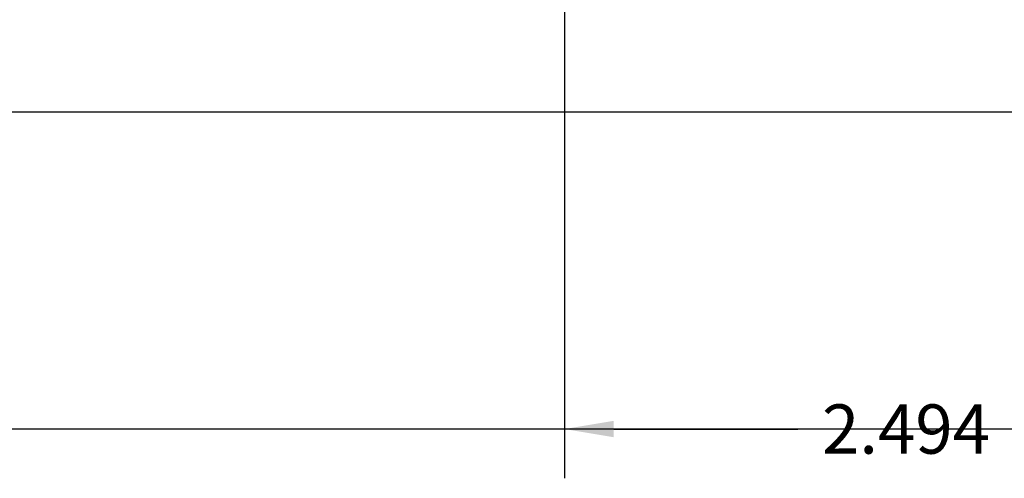
# Model space of a CAD drawing. Units: metres. Extents: x 4298.5 to 4325.2, y 2075 to 2095.8.
# Tile 21 of 35: x 4318.3 to 4321.9, y 2075 to 2076.7. Entities that reach past the tile are written whole.
import ezdxf

# ---------------------------------------------------------------- set-up
doc = ezdxf.new("R2010")
doc.units = ezdxf.units.M
doc.layers.add('A-ANNO-DIMS', color=2, linetype='Continuous', lineweight=18)
doc.styles.get("Standard").update_dxf_attribs({"font": 'arial.ttf'})
doc.dimstyles.get("Standard").update_dxf_attribs({"dimtxt": 0.18, "dimasz": 0.18, "dimexe": 0.18, "dimexo": 0.0625, "dimgap": 0.09, "dimtad": 0, "dimtih": 1, "dimtoh": 1, "dimdec": 4, "dimzin": 0, "dimdsep": 46, "dimtxsty": 'Standard', "dimcen": 0.09, "dimadec": 0, "dimazin": 0, "dimtfac": 1, "dimtdec": 4, "dimtofl": 0, "dimtmove": 0, "dimatfit": 3, "dimfxl": 1, "dimtolj": 1, "dimtzin": 0, "dimarcsym": 0})

# ---------------------------------------------------------------- blocks, each defined once
blk = doc.blocks.new('*D47')
at = {"layer": 'A-ANNO-DIMS', "color": 0, "lineweight": -2, "transparency": 16777216}
for p, q in [((4300.4306, 2084.4956), (4300.4306, 2074.9896)), ((4322.8106, 2084.4956), (4322.8106, 2074.9896)), ((4300.6106, 2075.1696), (4311.2252, 2075.1696)), ((4322.6306, 2075.1696), (4312.016, 2075.1696))]:
    blk.add_line(p, q, dxfattribs=at)
at = {"layer": 'A-ANNO-DIMS', "color": 0, "transparency": 16777216}
for points in [[(4300.6106, 2075.1996), (4300.6106, 2075.1396), (4300.4306, 2075.1696)], [(4322.6306, 2075.1996), (4322.6306, 2075.1396), (4322.8106, 2075.1696)]]:
    blk.add_solid(points, dxfattribs=at)
at = {"layer": 'Defpoints', "color": 0, "transparency": 16777216}
for p in [(4300.4306, 2084.5581), (4322.8106, 2084.5581), (4322.8106, 2075.1696)]:
    blk.add_point(p, dxfattribs=at)
at = {"layer": 'A-ANNO-DIMS', "color": 0, "transparency": 16777216, "insert": (4311.6206, 2075.1696), "char_height": 0.18, "attachment_point": 5}
blk.add_mtext('\\A1;22.38', dxfattribs=at)
blk = doc.blocks.new('*D48')
at = {"layer": 'A-ANNO-DIMS', "color": 0, "lineweight": -2, "transparency": 16777216}
for p, q in [((4310.1831, 2094.4781), (4324.7671, 2094.4781)), ((4324.5871, 2094.2981), (4324.5871, 2085.585)), ((4324.5871, 2076.5081), (4324.5871, 2085.2212)), ((4316.8731, 2076.3281), (4324.7671, 2076.3281))]:
    blk.add_line(p, q, dxfattribs=at)
at = {"layer": 'A-ANNO-DIMS', "color": 0, "transparency": 16777216}
for points in [[(4324.5571, 2094.2981), (4324.6171, 2094.2981), (4324.5871, 2094.4781)], [(4324.5571, 2076.5081), (4324.6171, 2076.5081), (4324.5871, 2076.3281)]]:
    blk.add_solid(points, dxfattribs=at)
at = {"layer": 'Defpoints', "color": 0, "transparency": 16777216}
for p in [(4310.1206, 2094.4781), (4316.8106, 2076.3281), (4324.5871, 2076.3281)]:
    blk.add_point(p, dxfattribs=at)
at = {"layer": 'A-ANNO-DIMS', "color": 0, "transparency": 16777216, "insert": (4324.5871, 2085.4031), "char_height": 0.18, "attachment_point": 5}
blk.add_mtext('\\A1;18.15', dxfattribs=at)
blk = doc.blocks.new('*D55')
at = {"layer": 'A-ANNO-DIMS', "color": 0, "lineweight": -2, "transparency": 16777216}
for p, q in [((4320.3167, 2084.4996), (4320.3167, 2074.9896)), ((4322.8106, 2084.4956), (4322.8106, 2074.9896)), ((4320.4967, 2075.1696), (4321.1688, 2075.1696)), ((4322.6306, 2075.1696), (4321.9585, 2075.1696))]:
    blk.add_line(p, q, dxfattribs=at)
at = {"layer": 'A-ANNO-DIMS', "color": 0, "transparency": 16777216}
for points in [[(4320.4967, 2075.1996), (4320.4967, 2075.1396), (4320.3167, 2075.1696)], [(4322.6306, 2075.1996), (4322.6306, 2075.1396), (4322.8106, 2075.1696)]]:
    blk.add_solid(points, dxfattribs=at)
at = {"layer": 'Defpoints', "color": 0, "transparency": 16777216}
for p in [(4320.3167, 2084.5621), (4322.8106, 2084.5581), (4322.8106, 2075.1696)]:
    blk.add_point(p, dxfattribs=at)
at = {"layer": 'A-ANNO-DIMS', "color": 0, "transparency": 16777216, "insert": (4321.5636, 2075.1696), "char_height": 0.18, "attachment_point": 5}
blk.add_mtext('\\A1;2.494', dxfattribs=at)

msp = doc.modelspace()

# ---------------------------------------------------------------- dimensions: what is measured, and where the dimension line sits
at = {"layer": 'A-ANNO-DIMS'}
dim = msp.add_linear_dim(base=(4324.5871, 2076.3281), p1=(4310.1206, 2094.4781), p2=(4316.8106, 2076.3281), angle=90, dimstyle='Standard', override={"dimdec": 2, "dimlfac": 1, "dimrnd": 0, "dimzin": 0, "dimdsep": 46, "dimlunit": 2}, dxfattribs=at)
dim.commit()
dim.dimension.update_dxf_attribs({"geometry": '*D48', "text_midpoint": (4324.5871, 2085.4031)})
for p1, override, picture, middle in [((4300.4306, 2084.5581), {"dimdec": 2, "dimlfac": 1, "dimrnd": 0, "dimzin": 0, "dimdsep": 46, "dimlunit": 2}, '*D47', (4311.6206, 2075.1696)), ((4320.3167, 2084.5621), {"dimdec": 3, "dimlfac": 1, "dimrnd": 0, "dimzin": 0, "dimdsep": 46, "dimlunit": 2}, '*D55', (4321.5636, 2075.1696))]:
    dim = msp.add_linear_dim(base=(4322.8106, 2075.1696), p1=p1, p2=(4322.8106, 2084.5581), dimstyle='Standard', override=override, dxfattribs=at)
    dim.commit()
    dim.dimension.update_dxf_attribs({"geometry": picture, "text_midpoint": middle})

doc.saveas('drawing.dxf')
